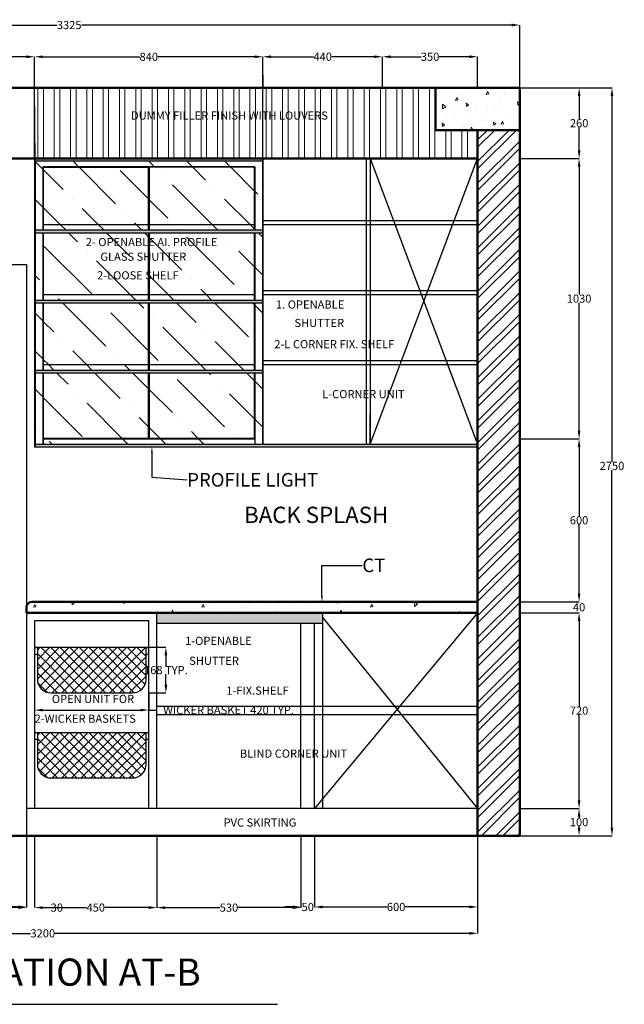
# Model space of a CAD drawing. Units: millimetres. Extents: x 26138 to 44889, y 15820 to 21179.
# Tile 6 of 8: x 37898 to 40122, y 15889 to 19510. Entities that reach past the tile are written whole.
import ezdxf
from ezdxf import colors
from ezdxf.entities.mleader import LeaderData, LeaderLine
from ezdxf.math import Vec2, Vec3

# ---------------------------------------------------------------- set-up
doc = ezdxf.new("R2010")
doc.units = ezdxf.units.MM
doc.header["$MEASUREMENT"] = 0
doc.header["$PDMODE"] = 3
for name, color, linetype, lineweight in [('A-ANNO-DIMS', 70, 'Continuous', 18), ('A-ANNO-SYMB', 1, 'Continuous', 18), ('A-ANNO-TEXT', 7, 'Continuous', 18), ('A-ELEV', 7, 'Continuous', 25), ('A-FURN-PATT', 40, 'Continuous', 13), ('A-WALL', 1, 'Continuous', 50), ('A-WALL-PATT', 8, 'Continuous', 13)]:
    doc.layers.add(name, color=color, linetype=linetype, lineweight=lineweight)
doc.styles.get("Standard").update_dxf_attribs({"font": 'arial.ttf'})
doc.dimstyles.get("Standard").update_dxf_attribs({"dimtxt": 30, "dimasz": 30, "dimexe": 0.18, "dimexo": 0.0625, "dimgap": 0.09, "dimtad": 0, "dimtih": 1, "dimtoh": 1, "dimdec": 0, "dimzin": 0, "dimdsep": 46, "dimtxsty": 'Standard', "dimcen": 0.09, "dimadec": 0, "dimazin": 0, "dimtfac": 1, "dimtdec": 0, "dimtofl": 0, "dimtmove": 0, "dimatfit": 3, "dimfxl": 1, "dimtolj": 1, "dimtzin": 0, "dimarcsym": 0})
pattern_1 = [(95, (-15.19, -1836.28), (88.24832, 74.04913), [12, -132]), (40, (-15.19, -1836.28), (-100.79875, 69.4029), [9.6, -105.6]), (145.45144, (-7.83, -1830.11), (-12.55043, 143.45204), [10.19843, -112.18274]), (91.1842, (-37.81, -1813.65), (139.47094, 102.0182), [18, -198]), (141.63564, (-26.19, -1805.15), (-4.464, 215.95387), [15.29765, -168.2742]), (36.18416, (-37.81, -1813.65), (-4.464, 215.9539), [14.4, -158.4]), (66, (-20.84, -1808), (113.08345, 21.9812), [12, -132]), (11, (-20.84, -1808), (-54.51337, 109.56935), [9.6, -105.6]), (116.45144, (-11.42, -1806.17), (58.57008, 131.55054), [10.19843, -112.18274]), (82.5, (-15.186, -1836.282), (-36.28691, 39.03837), [0, -104.32, 0, -107.2, 0, -106]), (52.5, (-15.186, -1836.28), (-14.85967, 74.38551), [0, -61.12, 0, -101.92, 0, -40.4]), (12.5, (-40.416, -1861.51), (62.946907, 57.84332), [0, -40, 0, -124.8, 0, -165.6]), (2.5, (-51.73, -1872.826), (54.6544, 77.30557), [0, -52, 0, -82.88, 0, -117.6])]
pattern_2 = [(135, (-15.19, -1836.28), (-192.02369, 52.3701), [246.875, -49.375, 0, -49.375])]

# ---------------------------------------------------------------- blocks, each defined once
blk = doc.blocks.new('*D73')
at = {"layer": 'A-ANNO-DIMS', "color": 0, "lineweight": -2, "transparency": 16777216}
for p, q in [((37102.5, 16508.7), (37102.5, 16246.8)), ((37922.5, 16508.7), (37922.5, 16246.8)), ((37132.5, 16247), (37479.3, 16247)), ((37892.5, 16247), (37545.7, 16247))]:
    blk.add_line(p, q, dxfattribs=at)
at = {"layer": 'A-ANNO-DIMS', "color": 0, "transparency": 16777216}
for points in [[(37132.5, 16252), (37132.5, 16242), (37102.5, 16247)], [(37892.5, 16252), (37892.5, 16242), (37922.5, 16247)]]:
    blk.add_solid(points, dxfattribs=at)
at = {"layer": 'Defpoints', "color": 0, "transparency": 16777216}
for p in [(37102.5, 16508.8), (37922.5, 16508.8), (37922.5, 16247)]:
    blk.add_point(p, dxfattribs=at)
at = {"layer": 'A-ANNO-DIMS', "color": 0, "transparency": 16777216, "insert": (37512.5, 16247), "char_height": 30, "attachment_point": 5}
blk.add_mtext('\\A1;820', dxfattribs=at)
blk = doc.blocks.new('*D74')
at = {"layer": 'A-ANNO-DIMS', "color": 0, "lineweight": -2, "transparency": 16777216}
for p, q in [((37922.5, 16508.7), (37922.5, 16244.3)), ((37952.5, 16508.7), (37952.5, 16244.3)), ((37892.5, 16244.5), (37862.5, 16244.5)), ((37982.5, 16244.5), (38012.5, 16244.5))]:
    blk.add_line(p, q, dxfattribs=at)
at = {"layer": 'A-ANNO-DIMS', "color": 0, "transparency": 16777216}
for points in [[(37892.5, 16249.5), (37892.5, 16239.5), (37922.5, 16244.5)], [(37982.5, 16249.5), (37982.5, 16239.5), (37952.5, 16244.5)]]:
    blk.add_solid(points, dxfattribs=at)
at = {"layer": 'Defpoints', "color": 0, "transparency": 16777216}
for p in [(37922.5, 16508.8), (37952.5, 16508.8), (37952.5, 16244.5)]:
    blk.add_point(p, dxfattribs=at)
at = {"layer": 'A-ANNO-DIMS', "color": 0, "transparency": 16777216, "insert": (38034.1, 16244.5), "char_height": 30, "attachment_point": 5}
blk.add_mtext('\\A1;30', dxfattribs=at)
blk = doc.blocks.new('*D75')
at = {"layer": 'A-ANNO-DIMS', "color": 0, "lineweight": -2, "transparency": 16777216}
for p, q in [((37952.5, 16508.7), (37952.5, 16244.3)), ((38402.5, 16508.7), (38402.5, 16244.3)), ((37982.5, 16244.5), (38143.8, 16244.5)), ((38372.5, 16244.5), (38211.3, 16244.5))]:
    blk.add_line(p, q, dxfattribs=at)
at = {"layer": 'A-ANNO-DIMS', "color": 0, "transparency": 16777216}
for points in [[(37982.5, 16249.5), (37982.5, 16239.5), (37952.5, 16244.5)], [(38372.5, 16249.5), (38372.5, 16239.5), (38402.5, 16244.5)]]:
    blk.add_solid(points, dxfattribs=at)
at = {"layer": 'Defpoints', "color": 0, "transparency": 16777216}
for p in [(37952.5, 16508.8), (38402.5, 16508.8), (38402.5, 16244.5)]:
    blk.add_point(p, dxfattribs=at)
at = {"layer": 'A-ANNO-DIMS', "color": 0, "transparency": 16777216, "insert": (38177.5, 16244.5), "char_height": 30, "attachment_point": 5}
blk.add_mtext('\\A1;450', dxfattribs=at)
blk = doc.blocks.new('*D76')
at = {"layer": 'A-ANNO-DIMS', "color": 0, "lineweight": -2, "transparency": 16777216}
for p, q in [((38402.5, 16508.7), (38402.5, 16244.1)), ((38932.5, 16508.7), (38932.5, 16244.1)), ((38432.5, 16244.3), (38634.4, 16244.3)), ((38902.5, 16244.3), (38700.7, 16244.3))]:
    blk.add_line(p, q, dxfattribs=at)
at = {"layer": 'A-ANNO-DIMS', "color": 0, "transparency": 16777216}
for points in [[(38432.5, 16249.3), (38432.5, 16239.3), (38402.5, 16244.3)], [(38902.5, 16249.3), (38902.5, 16239.3), (38932.5, 16244.3)]]:
    blk.add_solid(points, dxfattribs=at)
at = {"layer": 'Defpoints', "color": 0, "transparency": 16777216}
for p in [(38402.5, 16508.8), (38932.5, 16508.8), (38932.5, 16244.3)]:
    blk.add_point(p, dxfattribs=at)
at = {"layer": 'A-ANNO-DIMS', "color": 0, "transparency": 16777216, "insert": (38667.5, 16244.3), "char_height": 30, "attachment_point": 5}
blk.add_mtext('\\A1;530', dxfattribs=at)
blk = doc.blocks.new('*D77')
at = {"layer": 'A-ANNO-DIMS', "color": 0, "lineweight": -2, "transparency": 16777216}
for p, q in [((38932.5, 16508.7), (38932.5, 16246.6)), ((38982.5, 16508.7), (38982.5, 16246.6)), ((38902.5, 16246.8), (38872.5, 16246.8)), ((39012.5, 16246.8), (39042.5, 16246.8))]:
    blk.add_line(p, q, dxfattribs=at)
at = {"layer": 'A-ANNO-DIMS', "color": 0, "transparency": 16777216}
for points in [[(38902.5, 16251.8), (38902.5, 16241.8), (38932.5, 16246.8)], [(39012.5, 16251.8), (39012.5, 16241.8), (38982.5, 16246.8)]]:
    blk.add_solid(points, dxfattribs=at)
at = {"layer": 'Defpoints', "color": 0, "transparency": 16777216}
for p in [(38932.5, 16508.8), (38982.5, 16508.8), (38982.5, 16246.8)]:
    blk.add_point(p, dxfattribs=at)
at = {"layer": 'A-ANNO-DIMS', "color": 0, "transparency": 16777216, "insert": (38957.5, 16246.8), "char_height": 30, "attachment_point": 5}
blk.add_mtext('\\A1;50', dxfattribs=at)
blk = doc.blocks.new('*D78')
at = {"layer": 'A-ANNO-DIMS', "color": 0, "lineweight": -2, "transparency": 16777216}
for p, q in [((38982.5, 16508.7), (38982.5, 16246.6)), ((39582.5, 16508.7), (39582.5, 16246.6)), ((39012.5, 16246.8), (39249.3, 16246.8)), ((39552.5, 16246.8), (39315.8, 16246.8))]:
    blk.add_line(p, q, dxfattribs=at)
at = {"layer": 'A-ANNO-DIMS', "color": 0, "transparency": 16777216}
for points in [[(39012.5, 16251.8), (39012.5, 16241.8), (38982.5, 16246.8)], [(39552.5, 16251.8), (39552.5, 16241.8), (39582.5, 16246.8)]]:
    blk.add_solid(points, dxfattribs=at)
at = {"layer": 'Defpoints', "color": 0, "transparency": 16777216}
for p in [(38982.5, 16508.8), (39582.5, 16508.8), (39582.5, 16246.8)]:
    blk.add_point(p, dxfattribs=at)
at = {"layer": 'A-ANNO-DIMS', "color": 0, "transparency": 16777216, "insert": (39282.5, 16246.8), "char_height": 30, "attachment_point": 5}
blk.add_mtext('\\A1;600', dxfattribs=at)
blk = doc.blocks.new('*D79')
at = {"layer": 'A-ANNO-DIMS', "color": 0, "lineweight": -2, "transparency": 16777216}
for p, q in [((39737.6, 19258.8), (39956.1, 19258.8)), ((39955.9, 19228.8), (39955.9, 19144.2)), ((39955.9, 19028.8), (39955.9, 19113.4)), ((39737.6, 18998.8), (39956.1, 18998.8))]:
    blk.add_line(p, q, dxfattribs=at)
at = {"layer": 'A-ANNO-DIMS', "color": 0, "transparency": 16777216}
for points in [[(39950.9, 19228.8), (39960.9, 19228.8), (39955.9, 19258.8)], [(39950.9, 19028.8), (39960.9, 19028.8), (39955.9, 18998.8)]]:
    blk.add_solid(points, dxfattribs=at)
at = {"layer": 'Defpoints', "color": 0, "transparency": 16777216}
for p in [(39737.5, 19258.8), (39737.5, 18998.8), (39955.9, 18998.8)]:
    blk.add_point(p, dxfattribs=at)
at = {"layer": 'A-ANNO-DIMS', "color": 0, "transparency": 16777216, "insert": (39955.9, 19128.8), "char_height": 30, "attachment_point": 5}
blk.add_mtext('\\A1;260', dxfattribs=at)
blk = doc.blocks.new('*D80')
at = {"layer": 'A-ANNO-DIMS', "color": 0, "lineweight": -2, "transparency": 16777216}
for p, q in [((39737.6, 18998.8), (39955.9, 18998.8)), ((39955.7, 18968.8), (39955.7, 18499.2)), ((39955.7, 17998.8), (39955.7, 18468.3)), ((39737.6, 17968.8), (39955.9, 17968.8))]:
    blk.add_line(p, q, dxfattribs=at)
at = {"layer": 'A-ANNO-DIMS', "color": 0, "transparency": 16777216}
for points in [[(39950.7, 18968.8), (39960.7, 18968.8), (39955.7, 18998.8)], [(39950.7, 17998.8), (39960.7, 17998.8), (39955.7, 17968.8)]]:
    blk.add_solid(points, dxfattribs=at)
at = {"layer": 'Defpoints', "color": 0, "transparency": 16777216}
for p in [(39737.5, 18998.8), (39737.5, 17968.8), (39955.7, 17968.8)]:
    blk.add_point(p, dxfattribs=at)
at = {"layer": 'A-ANNO-DIMS', "color": 0, "transparency": 16777216, "insert": (39955.7, 18483.8), "char_height": 30, "attachment_point": 5}
blk.add_mtext('\\A1;1030', dxfattribs=at)
blk = doc.blocks.new('*D81')
at = {"layer": 'A-ANNO-DIMS', "color": 0, "lineweight": -2, "transparency": 16777216}
for p, q in [((39737.6, 17968.8), (39955.9, 17968.8)), ((39955.7, 17938.8), (39955.7, 17684.2)), ((39955.7, 17398.8), (39955.7, 17653.4)), ((39737.6, 17368.8), (39955.9, 17368.8))]:
    blk.add_line(p, q, dxfattribs=at)
at = {"layer": 'A-ANNO-DIMS', "color": 0, "transparency": 16777216}
for points in [[(39950.7, 17938.8), (39960.7, 17938.8), (39955.7, 17968.8)], [(39950.7, 17398.8), (39960.7, 17398.8), (39955.7, 17368.8)]]:
    blk.add_solid(points, dxfattribs=at)
at = {"layer": 'Defpoints', "color": 0, "transparency": 16777216}
for p in [(39737.5, 17968.8), (39737.5, 17368.8), (39955.7, 17368.8)]:
    blk.add_point(p, dxfattribs=at)
at = {"layer": 'A-ANNO-DIMS', "color": 0, "transparency": 16777216, "insert": (39955.7, 17668.8), "char_height": 30, "attachment_point": 5}
blk.add_mtext('\\A1;600', dxfattribs=at)
blk = doc.blocks.new('*D82')
at = {"layer": 'A-ANNO-DIMS', "color": 0, "lineweight": -2, "transparency": 16777216}
for p, q in [((39955.7, 17398.8), (39955.7, 17428.8)), ((39737.6, 17368.8), (39955.9, 17368.8)), ((39737.6, 17328.8), (39955.9, 17328.8)), ((39955.7, 17298.8), (39955.7, 17268.8))]:
    blk.add_line(p, q, dxfattribs=at)
at = {"layer": 'A-ANNO-DIMS', "color": 0, "transparency": 16777216}
for points in [[(39950.7, 17398.8), (39960.7, 17398.8), (39955.7, 17368.8)], [(39950.7, 17298.8), (39960.7, 17298.8), (39955.7, 17328.8)]]:
    blk.add_solid(points, dxfattribs=at)
at = {"layer": 'Defpoints', "color": 0, "transparency": 16777216}
for p in [(39737.5, 17368.8), (39737.5, 17328.8), (39955.7, 17328.8)]:
    blk.add_point(p, dxfattribs=at)
at = {"layer": 'A-ANNO-DIMS', "color": 0, "transparency": 16777216, "insert": (39955.7, 17348.8), "char_height": 30, "attachment_point": 5}
blk.add_mtext('\\A1;40', dxfattribs=at)
blk = doc.blocks.new('*D83')
at = {"layer": 'A-ANNO-DIMS', "color": 0, "lineweight": -2, "transparency": 16777216}
for p, q in [((39737.6, 17328.8), (39955.9, 17328.8)), ((39955.7, 17298.8), (39955.7, 16984.2)), ((39955.7, 16638.8), (39955.7, 16953.4)), ((39737.6, 16608.8), (39955.9, 16608.8))]:
    blk.add_line(p, q, dxfattribs=at)
at = {"layer": 'A-ANNO-DIMS', "color": 0, "transparency": 16777216}
for points in [[(39950.7, 17298.8), (39960.7, 17298.8), (39955.7, 17328.8)], [(39950.7, 16638.8), (39960.7, 16638.8), (39955.7, 16608.8)]]:
    blk.add_solid(points, dxfattribs=at)
at = {"layer": 'Defpoints', "color": 0, "transparency": 16777216}
for p in [(39737.5, 17328.8), (39737.5, 16608.8), (39955.7, 16608.8)]:
    blk.add_point(p, dxfattribs=at)
at = {"layer": 'A-ANNO-DIMS', "color": 0, "transparency": 16777216, "insert": (39955.7, 16968.8), "char_height": 30, "attachment_point": 5}
blk.add_mtext('\\A1;720', dxfattribs=at)
blk = doc.blocks.new('*D84')
at = {"layer": 'A-ANNO-DIMS', "color": 0, "lineweight": -2, "transparency": 16777216}
for p, q in [((39737.6, 16608.8), (39955.7, 16608.8)), ((39955.6, 16578.8), (39955.6, 16574.2)), ((39955.6, 16538.8), (39955.6, 16543.4)), ((39737.6, 16508.8), (39955.7, 16508.8))]:
    blk.add_line(p, q, dxfattribs=at)
at = {"layer": 'A-ANNO-DIMS', "color": 0, "transparency": 16777216}
for points in [[(39950.6, 16578.8), (39960.6, 16578.8), (39955.6, 16608.8)], [(39950.6, 16538.8), (39960.6, 16538.8), (39955.6, 16508.8)]]:
    blk.add_solid(points, dxfattribs=at)
at = {"layer": 'Defpoints', "color": 0, "transparency": 16777216}
for p in [(39737.5, 16608.8), (39737.5, 16508.8), (39955.6, 16508.8)]:
    blk.add_point(p, dxfattribs=at)
at = {"layer": 'A-ANNO-DIMS', "color": 0, "transparency": 16777216, "insert": (39955.6, 16558.8), "char_height": 30, "attachment_point": 5}
blk.add_mtext('\\A1;100', dxfattribs=at)
blk = doc.blocks.new('*D88')
at = {"layer": 'A-ANNO-DIMS', "color": 0, "lineweight": -2, "transparency": 16777216}
for p, q in [((36732.5, 19258.8), (36732.5, 19373.3)), ((36762.5, 19373.2), (37299.1, 19373.2)), ((37922.5, 19373.2), (37386, 19373.2)), ((37952.5, 19258.8), (37952.5, 19373.3))]:
    blk.add_line(p, q, dxfattribs=at)
at = {"layer": 'A-ANNO-DIMS', "color": 0, "transparency": 16777216}
for points in [[(36762.5, 19378.2), (36762.5, 19368.2), (36732.5, 19373.2)], [(37922.5, 19378.2), (37922.5, 19368.2), (37952.5, 19373.2)]]:
    blk.add_solid(points, dxfattribs=at)
at = {"layer": 'Defpoints', "color": 0, "transparency": 16777216}
for p in [(37952.5, 19373.2), (36732.5, 19258.8), (37952.5, 19258.8)]:
    blk.add_point(p, dxfattribs=at)
at = {"layer": 'A-ANNO-DIMS', "color": 0, "transparency": 16777216, "insert": (37342.5, 19373.2), "char_height": 30, "attachment_point": 5}
blk.add_mtext('\\A1;1220', dxfattribs=at)
blk = doc.blocks.new('*D89')
at = {"layer": 'A-ANNO-DIMS', "color": 0, "lineweight": -2, "transparency": 16777216}
for p, q in [((37952.5, 18998.8), (37952.5, 19373.3)), ((37982.5, 19373.2), (38339.3, 19373.2)), ((38762.5, 19373.2), (38405.7, 19373.2)), ((38792.5, 18998.8), (38792.5, 19373.3))]:
    blk.add_line(p, q, dxfattribs=at)
at = {"layer": 'A-ANNO-DIMS', "color": 0, "transparency": 16777216}
for points in [[(37982.5, 19378.2), (37982.5, 19368.2), (37952.5, 19373.2)], [(38762.5, 19378.2), (38762.5, 19368.2), (38792.5, 19373.2)]]:
    blk.add_solid(points, dxfattribs=at)
at = {"layer": 'Defpoints', "color": 0, "transparency": 16777216}
for p in [(38792.5, 19373.2), (37952.5, 18998.8), (38792.5, 18998.8)]:
    blk.add_point(p, dxfattribs=at)
at = {"layer": 'A-ANNO-DIMS', "color": 0, "transparency": 16777216, "insert": (38372.5, 19373.2), "char_height": 30, "attachment_point": 5}
blk.add_mtext('\\A1;840', dxfattribs=at)
blk = doc.blocks.new('*D90')
at = {"layer": 'A-ANNO-DIMS', "color": 0, "lineweight": -2, "transparency": 16777216}
for p, q in [((38792.5, 19258.8), (38792.5, 19373.5)), ((38822.5, 19373.3), (38978.8, 19373.3)), ((39202.5, 19373.3), (39046.3, 19373.3)), ((39232.5, 19258.8), (39232.5, 19373.5))]:
    blk.add_line(p, q, dxfattribs=at)
at = {"layer": 'A-ANNO-DIMS', "color": 0, "transparency": 16777216}
for points in [[(38822.5, 19378.3), (38822.5, 19368.3), (38792.5, 19373.3)], [(39202.5, 19378.3), (39202.5, 19368.3), (39232.5, 19373.3)]]:
    blk.add_solid(points, dxfattribs=at)
at = {"layer": 'Defpoints', "color": 0, "transparency": 16777216}
for p in [(39232.5, 19373.3), (38792.5, 19258.8), (39232.5, 19258.8)]:
    blk.add_point(p, dxfattribs=at)
at = {"layer": 'A-ANNO-DIMS', "color": 0, "transparency": 16777216, "insert": (39012.5, 19373.3), "char_height": 30, "attachment_point": 5}
blk.add_mtext('\\A1;440', dxfattribs=at)
blk = doc.blocks.new('*D91')
at = {"layer": 'A-ANNO-DIMS', "color": 0, "lineweight": -2, "transparency": 16777216}
for p, q in [((39232.5, 19258.8), (39232.5, 19373.5)), ((39262.5, 19373.3), (39374.4, 19373.3)), ((39552.5, 19373.3), (39440.7, 19373.3)), ((39582.5, 19258.8), (39582.5, 19373.5))]:
    blk.add_line(p, q, dxfattribs=at)
at = {"layer": 'A-ANNO-DIMS', "color": 0, "transparency": 16777216}
for points in [[(39262.5, 19378.3), (39262.5, 19368.3), (39232.5, 19373.3)], [(39552.5, 19378.3), (39552.5, 19368.3), (39582.5, 19373.3)]]:
    blk.add_solid(points, dxfattribs=at)
at = {"layer": 'Defpoints', "color": 0, "transparency": 16777216}
for p in [(39582.5, 19373.3), (39232.5, 19258.8), (39582.5, 19258.8)]:
    blk.add_point(p, dxfattribs=at)
at = {"layer": 'A-ANNO-DIMS', "color": 0, "transparency": 16777216, "insert": (39407.5, 19373.3), "char_height": 30, "attachment_point": 5}
blk.add_mtext('\\A1;350', dxfattribs=at)
blk = doc.blocks.new('*D92')
at = {"layer": 'A-ANNO-DIMS', "color": 0, "lineweight": -2, "transparency": 16777216}
for p, q in [((36382.5, 16509), (36382.5, 16149.6)), ((39582.5, 16508.7), (39582.5, 16149.6)), ((36412.5, 16149.8), (37937.7, 16149.8)), ((39552.5, 16149.8), (38027.4, 16149.8))]:
    blk.add_line(p, q, dxfattribs=at)
at = {"layer": 'A-ANNO-DIMS', "color": 0, "transparency": 16777216}
for points in [[(36412.5, 16154.8), (36412.5, 16144.8), (36382.5, 16149.8)], [(39552.5, 16154.8), (39552.5, 16144.8), (39582.5, 16149.8)]]:
    blk.add_solid(points, dxfattribs=at)
at = {"layer": 'Defpoints', "color": 0, "transparency": 16777216}
for p in [(36382.5, 16509), (39582.5, 16508.8), (39582.5, 16149.8)]:
    blk.add_point(p, dxfattribs=at)
at = {"layer": 'A-ANNO-DIMS', "color": 0, "transparency": 16777216, "insert": (37982.5, 16149.8), "char_height": 30, "attachment_point": 5}
blk.add_mtext('\\A1;3200', dxfattribs=at)
blk = doc.blocks.new('*D117')
at = {"layer": 'A-ANNO-DIMS', "color": 0, "lineweight": -2, "transparency": 16777216}
for p, q in [((39737.6, 19258.8), (40076.9, 19258.8)), ((40076.7, 19228.8), (40076.7, 17884.2)), ((40076.7, 16538.8), (40076.7, 17853.3)), ((39737.6, 16508.8), (40076.9, 16508.8))]:
    blk.add_line(p, q, dxfattribs=at)
at = {"layer": 'A-ANNO-DIMS', "color": 0, "transparency": 16777216}
for points in [[(40071.7, 19228.8), (40081.7, 19228.8), (40076.7, 19258.8)], [(40071.7, 16538.8), (40081.7, 16538.8), (40076.7, 16508.8)]]:
    blk.add_solid(points, dxfattribs=at)
at = {"layer": 'Defpoints', "color": 0, "transparency": 16777216}
for p in [(39737.5, 19258.8), (39737.5, 16508.8), (40076.7, 16508.8)]:
    blk.add_point(p, dxfattribs=at)
at = {"layer": 'A-ANNO-DIMS', "color": 0, "transparency": 16777216, "insert": (40076.7, 17868.7), "char_height": 30, "attachment_point": 5}
blk.add_mtext('\\A1;2750', dxfattribs=at)
blk = doc.blocks.new('*D118')
at = {"layer": 'A-ANNO-DIMS', "color": 0, "lineweight": -2, "transparency": 16777216}
for p, q in [((36412.5, 19258.8), (36412.5, 19490)), ((36442.5, 19489.9), (38034.6, 19489.9)), ((39707.5, 19489.9), (38124.6, 19489.9)), ((39737.5, 19258.8), (39737.5, 19490))]:
    blk.add_line(p, q, dxfattribs=at)
at = {"layer": 'A-ANNO-DIMS', "color": 0, "transparency": 16777216}
for points in [[(36442.5, 19494.9), (36442.5, 19484.9), (36412.5, 19489.9)], [(39707.5, 19494.9), (39707.5, 19484.9), (39737.5, 19489.9)]]:
    blk.add_solid(points, dxfattribs=at)
at = {"layer": 'Defpoints', "color": 0, "transparency": 16777216}
for p in [(39737.5, 19489.9), (36412.5, 19258.8), (39737.5, 19258.8)]:
    blk.add_point(p, dxfattribs=at)
at = {"layer": 'A-ANNO-DIMS', "color": 0, "transparency": 16777216, "insert": (38079.6, 19489.9), "char_height": 30, "attachment_point": 5}
blk.add_mtext('\\A1;3325', dxfattribs=at)
blk = doc.blocks.new('WICKER-BASKET')
for p, q in [((0, 167.7), (10, 167.7)), ((10, 167.7), (10, 50)), ((410, 50), (410, 167.7)), ((410, 167.7), (420, 167.7)), ((60, 0), (360, 0))]:
    blk.add_line(p, q)
for centre, start, end in [((60, 50), 180, 270), ((360, 50), 270, 0)]:
    blk.add_arc(centre, 50, start, end)
blk = doc.blocks.new('*D129')
at = {"layer": 'A-ANNO-DIMS', "color": 0, "lineweight": -2, "transparency": 16777216}
for p, q in [((37952.5, 17033.7), (37952.5, 16970.6)), ((38372.5, 17033.7), (38372.5, 16970.6)), ((37982.5, 16970.8), (38342.5, 16970.8)), ((38372.5, 16970.8), (38402.5, 16970.8))]:
    blk.add_line(p, q, dxfattribs=at)
at = {"layer": 'A-ANNO-DIMS', "color": 0, "transparency": 16777216}
for points in [[(37982.5, 16975.8), (37982.5, 16965.8), (37952.5, 16970.8)], [(38342.5, 16975.8), (38342.5, 16965.8), (38372.5, 16970.8)]]:
    blk.add_solid(points, dxfattribs=at)
at = {"layer": 'Defpoints', "color": 0, "transparency": 16777216}
for p in [(37952.5, 17033.8), (38372.5, 17033.8), (38372.5, 16970.8)]:
    blk.add_point(p, dxfattribs=at)
at = {"layer": 'A-ANNO-DIMS', "color": 0, "transparency": 16777216, "insert": (38666.1, 16970.8), "char_height": 30, "attachment_point": 5}
blk.add_mtext('\\A1;WICKER BASKET 420 TYP.', dxfattribs=at)
blk = doc.blocks.new('*D130')
at = {"layer": 'A-ANNO-DIMS', "color": 0, "lineweight": -2, "transparency": 16777216}
for p, q in [((38372.6, 17201.6), (38435.7, 17201.6)), ((38435.5, 17171.6), (38435.5, 17133.1)), ((38435.5, 17063.8), (38435.5, 17102.3)), ((38372.6, 17033.8), (38435.7, 17033.8))]:
    blk.add_line(p, q, dxfattribs=at)
at = {"layer": 'A-ANNO-DIMS', "color": 0, "transparency": 16777216}
for points in [[(38430.5, 17171.6), (38440.5, 17171.6), (38435.5, 17201.6)], [(38430.5, 17063.8), (38440.5, 17063.8), (38435.5, 17033.8)]]:
    blk.add_solid(points, dxfattribs=at)
at = {"layer": 'Defpoints', "color": 0, "transparency": 16777216}
for p in [(38372.5, 17201.6), (38435.5, 17201.6), (38372.5, 17033.8)]:
    blk.add_point(p, dxfattribs=at)
at = {"layer": 'A-ANNO-DIMS', "color": 0, "transparency": 16777216, "insert": (38435.5, 17117.7), "char_height": 30, "attachment_point": 5}
blk.add_mtext('\\A1;168 TYP.', dxfattribs=at)

msp = doc.modelspace()

# ---------------------------------------------------------------- hatches: boundary and pattern name
at = {"layer": 'A-FURN-PATT'}
h = msp.add_hatch(color=256, dxfattribs=at)
h.dxf.hatch_style = 1
h.paths.add_polyline_path([(38792.548, 18988.766), (38792.548, 18998.766), (37952.548, 18998.766), (37952.548, 18988.766)])
h = msp.add_hatch(dxfattribs=at)
h.set_pattern_fill('ANSI36', color=256, scale=790, angle=90)
h.set_pattern_definition(pattern_2)
h.paths.add_polyline_path([(37982.548, 18968.766), (38762.548, 18968.766), (38762.548, 18736.288), (38790.548, 18736.288), (38790.548, 18988.766), (37954.548, 18988.766), (37954.548, 18736.288), (37982.548, 18736.288)])
h = msp.add_hatch(dxfattribs=at)
h.set_pattern_fill('ANSI36', color=256, scale=790, angle=90)
h.set_pattern_definition(pattern_2)
h.paths.add_polyline_path([(37984.548, 18966.766), (37984.548, 18756.266), (38370.548, 18756.266), (38370.548, 18966.766)], flags=17)
h = msp.add_hatch(dxfattribs=at)
h.set_pattern_fill('ANSI36', color=256, scale=790, angle=90)
h.set_pattern_definition(pattern_2)
h.paths.add_polyline_path([(38374.548, 18966.766), (38374.548, 18756.266), (38760.548, 18756.266), (38760.548, 18966.766)], flags=17)
h = msp.add_hatch(dxfattribs=at)
h.set_pattern_fill('ANSI36', color=256, scale=790, angle=90)
h.set_pattern_definition(pattern_2)
h.paths.add_polyline_path([(38370.548, 18756.266), (37984.548, 18756.266), (37984.548, 18736.288), (38370.548, 18736.288)], flags=17)
h = msp.add_hatch(dxfattribs=at)
h.set_pattern_fill('ANSI36', color=256, scale=790, angle=90)
h.set_pattern_definition(pattern_2)
h.paths.add_polyline_path([(38760.548, 18756.266), (38374.548, 18756.266), (38374.548, 18736.288), (38760.548, 18736.288)], flags=17)
h = msp.add_hatch(color=256, dxfattribs=at)
h.dxf.hatch_style = 1
h.paths.add_polyline_path([(37952.548, 18736.288), (37952.548, 18726.266), (38792.548, 18726.266), (38792.548, 18736.288)])
h = msp.add_hatch(dxfattribs=at)
h.set_pattern_fill('ANSI36', color=256, scale=790, angle=90)
h.set_pattern_definition(pattern_2)
h.paths.add_polyline_path([(37982.548, 18726.266), (37954.548, 18726.266), (37954.548, 18478.766), (37982.548, 18478.766)])
h = msp.add_hatch(dxfattribs=at)
h.set_pattern_fill('ANSI36', color=256, scale=790, angle=90)
h.set_pattern_definition(pattern_2)
h.paths.add_polyline_path([(38370.548, 18498.766), (38370.548, 18726.266), (37984.548, 18726.266), (37984.548, 18498.766)])
h = msp.add_hatch(dxfattribs=at)
h.set_pattern_fill('ANSI36', color=256, scale=790, angle=90)
h.set_pattern_definition(pattern_2)
h.paths.add_polyline_path([(38760.548, 18498.766), (38760.548, 18726.266), (38374.548, 18726.266), (38374.548, 18498.766)])
h = msp.add_hatch(dxfattribs=at)
h.set_pattern_fill('ANSI36', color=256, scale=790, angle=90)
h.set_pattern_definition(pattern_2)
h.paths.add_polyline_path([(38790.548, 18726.266), (38762.548, 18726.266), (38762.548, 18478.766), (38790.548, 18478.766)])
h = msp.add_hatch(color=256, dxfattribs=at)
h.dxf.hatch_style = 1
h.paths.add_polyline_path([(37952.548, 18478.766), (37952.548, 18468.766), (38792.548, 18468.766), (38792.548, 18478.766)])
h = msp.add_hatch(dxfattribs=at)
h.set_pattern_fill('ANSI36', color=256, scale=790, angle=90)
h.set_pattern_definition(pattern_2)
h.paths.add_polyline_path([(37982.548, 18468.766), (37954.548, 18468.766), (37954.548, 18221.266), (37982.548, 18221.266)])
h = msp.add_hatch(dxfattribs=at)
h.set_pattern_fill('ANSI36', color=256, scale=790, angle=90)
h.set_pattern_definition(pattern_2)
h.paths.add_polyline_path([(38370.548, 18498.766), (37984.548, 18498.766), (37984.548, 18478.766), (38370.548, 18478.766)])
h = msp.add_hatch(dxfattribs=at)
h.set_pattern_fill('ANSI36', color=256, scale=790, angle=90)
h.set_pattern_definition(pattern_2)
h.paths.add_polyline_path([(38370.548, 18241.266), (38370.548, 18468.766), (37984.548, 18468.766), (37984.548, 18241.266)])
h = msp.add_hatch(dxfattribs=at)
h.set_pattern_fill('ANSI36', color=256, scale=790, angle=90)
h.set_pattern_definition(pattern_2)
h.paths.add_polyline_path([(38760.548, 18498.766), (38374.548, 18498.766), (38374.548, 18478.766), (38760.548, 18478.766)])
h = msp.add_hatch(dxfattribs=at)
h.set_pattern_fill('ANSI36', color=256, scale=790, angle=90)
h.set_pattern_definition(pattern_2)
h.paths.add_polyline_path([(38374.548, 18468.766), (38374.548, 18241.266), (38760.548, 18241.266), (38760.548, 18468.766)])
h = msp.add_hatch(dxfattribs=at)
h.set_pattern_fill('ANSI36', color=256, scale=790, angle=90)
h.set_pattern_definition(pattern_2)
h.paths.add_polyline_path([(38790.548, 18468.766), (38762.548, 18468.766), (38762.548, 18221.266), (38790.548, 18221.266)])
h = msp.add_hatch(color=256, dxfattribs=at)
h.dxf.hatch_style = 1
h.paths.add_polyline_path([(38792.548, 18211.266), (38792.548, 18221.266), (37952.548, 18221.266), (37952.548, 18211.266)])
h = msp.add_hatch(dxfattribs=at)
h.set_pattern_fill('ANSI36', color=256, scale=790, angle=90)
h.set_pattern_definition(pattern_2)
h.paths.add_polyline_path([(38370.548, 18241.266), (37984.548, 18241.266), (37984.548, 18221.266), (38370.548, 18221.266)])
h = msp.add_hatch(dxfattribs=at)
h.set_pattern_fill('ANSI36', color=256, scale=790, angle=90)
h.set_pattern_definition(pattern_2)
h.paths.add_polyline_path([(38760.548, 18241.266), (38374.548, 18241.266), (38374.548, 18221.266), (38760.548, 18221.266)])
h = msp.add_hatch(dxfattribs=at)
h.set_pattern_fill('ANSI36', color=256, scale=790, angle=90)
h.set_pattern_definition(pattern_2)
h.paths.add_polyline_path([(37982.548, 18211.266), (37954.548, 18211.266), (37954.548, 17948.766), (37982.548, 17948.766)])
h = msp.add_hatch(dxfattribs=at)
h.set_pattern_fill('ANSI36', color=256, scale=790, angle=90)
h.set_pattern_definition(pattern_2)
h.paths.add_polyline_path([(37984.548, 18211.266), (37984.548, 17970.766), (38370.548, 17970.766), (38370.548, 18211.266)])
h = msp.add_hatch(dxfattribs=at)
h.set_pattern_fill('ANSI36', color=256, scale=790, angle=90)
h.set_pattern_definition(pattern_2)
h.paths.add_polyline_path([(38374.548, 18211.266), (38374.548, 17970.766), (38760.548, 17970.766), (38760.548, 18211.266)])
h = msp.add_hatch(dxfattribs=at)
h.set_pattern_fill('ANSI36', color=256, scale=790, angle=90)
h.set_pattern_definition(pattern_2)
h.paths.add_polyline_path([(38790.548, 18211.266), (38762.548, 18211.266), (38762.548, 17948.766), (38790.548, 17948.766)])
h = msp.add_hatch(dxfattribs=at)
h.set_pattern_fill('ANSI36', color=256, scale=790, angle=90)
h.set_pattern_definition(pattern_2)
h.paths.add_polyline_path([(38762.548, 17968.766), (37984.548, 17968.766), (37984.548, 17948.766), (38762.548, 17948.766)])
h = msp.add_hatch(color=256, dxfattribs=at)
h.dxf.hatch_style = 1
h.paths.add_polyline_path([(37952.548, 17948.766), (37952.548, 17938.766), (38792.548, 17938.766), (38792.548, 17948.766)])
h = msp.add_hatch(color=256, dxfattribs=at)
h.dxf.hatch_style = 1
h.paths.add_polyline_path([(39582.548, 17948.766), (37952.548, 17948.766), (37952.548, 17938.766), (39582.548, 17938.766)])
h = msp.add_hatch(color=256, dxfattribs=at)
h.dxf.hatch_style = 1
h.paths.add_polyline_path([(39552.548, 17948.766), (38792.548, 17948.766), (38792.548, 17938.766), (39552.548, 17938.766)])
h = msp.add_hatch(color=256, dxfattribs=at)
h.dxf.hatch_style = 1
h.paths.add_polyline_path([(38402.548, 17328.766), (38402.548, 17288.766), (39012.548, 17288.766), (39012.548, 17328.766)])
h = msp.add_hatch(dxfattribs=at)
h.set_pattern_fill('ANSI37', color=256, scale=200, angle=90)
h.set_pattern_definition([(135, (-15.186, -1836.282), (-17.67767, -17.67767), []), (225, (-15.186, -1836.282), (17.67767, -17.67767), [])])
h.paths.add_polyline_path([(38312.548, 17033.811, 0.41421356), (38362.548, 17083.811), (38362.548, 17201.557), (37962.548, 17201.557), (37962.548, 17083.811, 0.41421356), (38012.548, 17033.811)])
h = msp.add_hatch(dxfattribs=at)
h.set_pattern_fill('ANSI37', color=256, scale=200, angle=90)
h.set_pattern_definition([(135, (-15.186, -2148.976), (-17.67767, -17.67767), []), (225, (-15.186, -2148.976), (17.67767, -17.67767), [])])
h.paths.add_polyline_path([(38312.548, 16721.117, 0.41421356), (38362.548, 16771.117), (38362.548, 16888.863), (37962.548, 16888.863), (37962.548, 16771.117, 0.41421356), (38012.548, 16721.117)])
at = {"layer": 'A-WALL-PATT'}
h = msp.add_hatch(dxfattribs=at)
h.set_pattern_fill('ANSI32', color=256, scale=160, angle=45)
h.set_pattern_definition([(90, (-15.186, -1836.28), (-60, 0), []), (90, (4.814, -1816.28), (-60, 0), [])])
h.paths.add_polyline_path([(37952.548, 19258.766), (37954.474, 18998.766), (39582.548, 18998.766), (39582.548, 19103.766), (39427.548, 19103.766), (39427.548, 19258.766)])
h.paths.add_polyline_path([(38299.413, 19133.795), (39106.641, 19133.795), (39106.641, 19180.36), (38299.413, 19180.36)], flags=24)
h = msp.add_hatch(dxfattribs=at)
h.set_pattern_fill('AR-CONC', color=256, scale=16, angle=45)
h.set_pattern_definition(pattern_1)
h.paths.add_polyline_path([(39737.548, 19103.766), (39737.548, 19258.766), (39427.548, 19258.766), (39427.548, 19103.766)])
h = msp.add_hatch(dxfattribs=at)
h.set_pattern_fill('ANSI32', color=256, scale=150)
h.set_pattern_definition([(45, (-15.186, -1836.28), (-39.774756, 39.774756), []), (45, (11.33, -1836.28), (-39.774756, 39.774756), [])])
h.paths.add_polyline_path([(39737.548, 19103.766), (39582.548, 19103.766), (39582.548, 16508.766), (39737.548, 16508.766)])
h = msp.add_hatch(dxfattribs=at)
h.set_pattern_fill('AR-CONC', color=256, scale=16, angle=45)
h.set_pattern_definition(pattern_1)
h.paths.add_polyline_path([(37942.548, 17368.766, 0.41421356), (37922.548, 17348.766), (37922.548, 17328.766), (38402.548, 17328.766), (39582.548, 17328.766), (39582.548, 17368.766)])

# ---------------------------------------------------------------- linework, layer by layer
at = {"layer": 'A-ANNO-SYMB'}
for p in [(37952.548, 18741.266), (37952.548, 18483.766), (37952.548, 18226.266)]:
    msp.add_point(p, dxfattribs=at)
at = {"layer": 'A-ELEV'}
for p, q in [((38792.548, 19306.068), (38792.548, 19258.766)), ((37954.548, 18988.766), (37952.548, 19258.766)), ((37952.548, 18998.766), (37952.548, 17938.766)), ((38792.548, 18988.766), (37952.548, 18988.766)), ((37954.548, 18998.766), (37954.548, 17938.766)), ((38790.548, 18998.766), (38790.548, 17948.766)), ((38792.548, 18998.766), (38792.548, 17948.766)), ((39172.548, 18998.766), (39172.548, 17948.766)), ((39187.548, 18998.766), (39187.548, 17948.766)), ((39187.548, 18998.766), (39582.548, 17948.766)), ((39187.548, 17948.766), (39582.548, 18998.766)), ((37982.548, 18968.766), (37982.548, 18736.288)), ((38762.548, 18968.766), (37982.548, 18968.766)), ((37984.548, 18966.766), (37984.548, 18736.288)), ((37984.548, 18966.766), (38370.548, 18966.766)), ((38370.548, 18966.766), (38370.548, 18736.266)), ((38374.548, 18966.766), (38374.548, 18736.266)), ((38760.548, 18966.766), (38374.548, 18966.766)), ((38760.548, 18966.766), (38760.548, 18736.288)), ((38762.548, 18968.766), (38762.548, 18736.288)), ((37982.548, 18756.266), (38762.548, 18756.266)), ((38792.548, 18771.266), (39582.548, 18771.266)), ((38792.548, 18756.266), (39582.548, 18756.266)), ((37952.548, 18736.288), (38792.548, 18736.288)), ((37952.548, 18726.266), (38792.548, 18726.266)), ((37982.548, 18726.266), (37982.548, 18478.766)), ((37984.548, 18726.266), (37984.548, 18478.766)), ((38370.548, 18726.266), (38370.548, 18478.766)), ((38374.548, 18726.266), (38374.548, 18478.766)), ((38760.548, 18726.266), (38760.548, 18478.766)), ((38762.548, 18726.266), (38762.548, 18478.766)), ((37102.548, 18608.766), (37922.548, 18608.766)), ((37922.548, 18608.766), (37922.548, 16508.766)), ((38792.548, 18513.766), (39582.548, 18513.766)), ((37952.548, 18478.766), (38792.548, 18478.766)), ((37952.548, 18468.766), (38792.548, 18468.766)), ((37982.548, 18498.766), (38762.548, 18498.766)), ((37982.548, 18468.766), (37982.548, 18221.266)), ((37984.548, 18468.766), (37984.548, 18221.266)), ((38370.548, 18468.766), (38370.548, 18221.266)), ((38374.548, 18468.766), (38374.548, 18221.266)), ((38760.548, 18468.766), (38760.548, 18221.266)), ((38762.548, 18468.766), (38762.548, 18221.266)), ((38792.548, 18498.766), (39582.548, 18498.766)), ((38792.548, 18256.266), (39582.548, 18256.266)), ((37952.548, 18221.266), (38792.548, 18221.266)), ((37982.548, 18241.266), (38762.548, 18241.266)), ((38792.548, 18241.266), (39582.548, 18241.266)), ((37952.548, 18211.266), (38792.548, 18211.266)), ((37982.548, 18211.266), (37982.548, 17948.766)), ((37984.548, 18211.266), (37984.548, 17948.766)), ((38370.548, 18211.266), (38370.548, 17968.766)), ((38374.548, 18211.266), (38374.548, 17968.766)), ((38760.548, 18211.266), (38760.548, 17970.766)), ((38762.548, 18211.266), (38762.548, 17948.766)), ((39187.548, 17948.766), (39187.548, 18057.233)), ((37982.548, 17968.766), (38762.548, 17968.766)), ((37984.548, 17970.766), (38760.548, 17970.766)), ((37952.548, 17948.766), (39582.548, 17948.766)), ((37952.548, 17938.766), (39582.548, 17938.766)), ((39172.548, 17948.766), (39187.548, 17948.766)), ((37922.548, 17313.766), (37922.548, 16608.766)), ((38402.548, 16953.766), (38402.548, 17328.766)), ((39582.548, 17328.766), (38982.548, 16608.766)), ((39012.548, 16608.766), (39012.548, 17328.766)), ((39012.548, 17310.304), (39582.548, 16608.766)), ((37952.548, 17298.766), (37952.548, 16608.766)), ((38372.548, 17298.766), (37952.548, 17298.766)), ((38372.548, 16608.766), (38372.548, 17298.766)), ((39012.548, 17288.766), (38402.548, 17288.766)), ((38932.548, 16608.766), (38932.548, 17288.766)), ((38982.548, 16608.766), (38982.548, 17288.766)), ((37957.548, 17201.557), (38367.548, 17201.557)), ((37952.548, 17176.823), (37962.548, 17176.823)), ((38362.548, 17176.823), (38372.548, 17176.823)), ((38372.548, 17033.811), (38372.548, 17033.811)), ((39582.548, 16983.766), (38402.548, 16983.766)), ((38372.548, 16608.766), (38372.548, 16958.766)), ((38402.548, 16608.766), (38402.548, 16958.766)), ((39582.548, 16953.766), (38402.548, 16953.766)), ((37957.548, 16888.863), (38367.548, 16888.863)), ((37952.548, 16864.129), (37962.548, 16864.129)), ((38362.548, 16864.129), (38372.548, 16864.129)), ((38372.548, 16721.117), (38372.548, 16721.117)), ((39582.548, 16608.766), (37922.548, 16608.766)), ((36832.787, 15888.819), (38846.464, 15888.819))]:
    msp.add_line(p, q, dxfattribs=at)
at = {"layer": 'A-WALL'}
for p, q in [((39737.548, 19258.766), (36109.548, 19258.766)), ((39427.548, 19103.766), (39427.548, 19258.766)), ((39737.548, 16508.766), (39737.548, 19258.766)), ((39737.548, 19258.766), (39737.548, 19103.766)), ((39737.548, 19103.766), (39427.548, 19103.766)), ((39582.548, 16508.766), (39582.548, 19103.766)), ((39582.548, 18998.766), (36109.548, 18998.766)), ((37922.548, 17348.766), (37922.548, 17328.766)), ((39582.548, 17368.766), (37942.548, 17368.766)), ((39582.548, 17328.766), (37922.548, 17328.766)), ((36109.548, 16508.766), (39737.548, 16508.766))]:
    msp.add_line(p, q, dxfattribs=at)
msp.add_arc((37942.548, 17348.766), 20, 90, 180, dxfattribs=at)

# ---------------------------------------------------------------- block references
at = {"layer": 'A-ELEV'}
for p in [(37952.548, 17033.811), (37952.548, 16721.117)]:
    msp.add_blockref('WICKER-BASKET', p, dxfattribs=at)

# ---------------------------------------------------------------- texts
at = {"layer": 'A-ANNO-TEXT'}
for s, height, p in [('DUMMY FILLER FINISH WITH LOUVERS', 30, (38307.174, 19142.067)), ('2- OPENABLE AI. PROFILE', 30, (38140.677, 18676.74)), ('GLASS SHUTTER', 30, (38194.438, 18622.978)), ('2-LOOSE SHELF', 30, (38182.123, 18554.457)), ('1. OPENABLE', 30, (38840.54, 18447.13)), ('SHUTTER', 30, (38908.377, 18379.409)), ('2-L CORNER FIX. SHELF', 30, (38834.352, 18301.377)), ('L-CORNER UNIT', 30, (39010.624, 18117.605)), ('BACK SPLASH', 60, (38723.173, 17658.639)), ('1-OPENABLE', 30, (38506.071, 17210.266)), ('SHUTTER', 30, (38521.321, 17137.114)), ('1-FIX.SHELF', 30, (38657.74, 17027.386)), ('OPEN UNIT FOR ', 30, (38015.758, 16996.744)), ('2-WICKER BASKETS', 30, (37952.548, 16924.235)), ('BLIND CORNER UNIT', 30, (38707.74, 16795.739)), ('PVC SKIRTING', 30, (38647.633, 16542.267)), ('KITCHEN ELEVATION AT-B', 100, (36907.79, 15957.078))]:
    msp.add_text(s, height=height, dxfattribs=at).set_placement(p)

# ---------------------------------------------------------------- dimensions: what is measured, and where the dimension line sits
at = {"layer": 'A-ANNO-DIMS'}
dim = msp.add_linear_dim(base=(39737.548, 19489.858), p1=(36412.548, 19258.766), p2=(39737.548, 19258.766), dimstyle='Standard', override={"dimclrd": 0, "dimclre": 0, "dimclrt": 0}, dxfattribs=at)
dim.commit()
dim.dimension.update_dxf_attribs({"geometry": '*D118', "text_midpoint": (38079.614, 19489.858), "dimtype": 160})
for base, p1, p2, picture, middle in [((37952.548, 19373.162), (36732.548, 19258.766), (37952.548, 19258.766), '*D88', (37342.548, 19373.162)), ((38792.548, 19373.162), (37952.548, 18998.766), (38792.548, 18998.766), '*D89', (38372.548, 19373.162)), ((39232.548, 19373.342), (38792.548, 19258.766), (39232.548, 19258.766), '*D90', (39012.548, 19373.342)), ((39582.548, 19373.342), (39232.548, 19258.766), (39582.548, 19258.766), '*D91', (39407.548, 19373.342)), ((39582.548, 16149.822), (36382.548, 16509.017), (39582.548, 16508.766), '*D92', (37982.548, 16149.822)), ((37922.548, 16246.967), (37102.548, 16508.766), (37922.548, 16508.766), '*D73', (37512.548, 16246.967)), ((37952.548, 16244.467), (37922.548, 16508.766), (37952.548, 16508.766), '*D74', (38034.064, 16244.467)), ((38402.548, 16244.467), (37952.548, 16508.766), (38402.548, 16508.766), '*D75', (38177.548, 16244.467)), ((38932.548, 16244.287), (38402.548, 16508.766), (38932.548, 16508.766), '*D76', (38667.548, 16244.287)), ((38982.548, 16246.787), (38932.548, 16508.766), (38982.548, 16508.766), '*D77', (38957.548, 16246.787)), ((39582.548, 16246.787), (38982.548, 16508.766), (39582.548, 16508.766), '*D78', (39282.548, 16246.787))]:
    dim = msp.add_linear_dim(base=base, p1=p1, p2=p2, dimstyle='Standard', override={"dimclrd": 0, "dimclre": 0, "dimclrt": 0}, dxfattribs=at)
    dim.commit()
    dim.dimension.update_dxf_attribs({"geometry": picture, "text_midpoint": middle})
for base, p1, p2, picture, middle in [((39955.919, 18998.766), (39737.548, 19258.766), (39737.548, 18998.766), '*D79', (39955.919, 19128.766)), ((39955.739, 17968.766), (39737.548, 18998.766), (39737.548, 17968.766), '*D80', (39955.739, 18483.766)), ((39955.739, 17368.766), (39737.548, 17968.766), (39737.548, 17368.766), '*D81', (39955.739, 17668.766)), ((39955.739, 17328.766), (39737.548, 17368.766), (39737.548, 17328.766), '*D82', (39955.739, 17348.766)), ((39955.739, 16608.766), (39737.548, 17328.766), (39737.548, 16608.766), '*D83', (39955.739, 16968.766)), ((39955.559, 16508.766), (39737.548, 16608.766), (39737.548, 16508.766), '*D84', (39955.559, 16558.766))]:
    dim = msp.add_linear_dim(base=base, p1=p1, p2=p2, angle=90, dimstyle='Standard', override={"dimclrd": 0, "dimclre": 0, "dimclrt": 0}, dxfattribs=at)
    dim.commit()
    dim.dimension.update_dxf_attribs({"geometry": picture, "text_midpoint": middle})
dim = msp.add_linear_dim(base=(40076.692, 16508.766), p1=(39737.548, 19258.766), p2=(39737.548, 16508.766), angle=90, dimstyle='Standard', override={"dimclrd": 0, "dimclre": 0, "dimclrt": 0}, dxfattribs=at)
dim.commit()
dim.dimension.update_dxf_attribs({"geometry": '*D117', "text_midpoint": (40076.692, 17868.746), "dimtype": 160})
dim = msp.add_linear_dim(base=(38435.548, 17201.557), p1=(38372.548, 17033.811), p2=(38372.548, 17201.557), angle=90, text='<> TYP.', dimstyle='Standard', override={"dimdec": 0, "dimrnd": 0, "dimzin": 0, "dimlunit": 2}, dxfattribs=at)
dim.commit()
dim.dimension.update_dxf_attribs({"geometry": '*D130', "text_midpoint": (38435.548, 17117.684)})
dim = msp.add_linear_dim(base=(38372.548, 16970.811), p1=(37952.548, 17033.811), p2=(38372.548, 17033.811), text='WICKER BASKET <> TYP.', dimstyle='Standard', override={"dimdec": 0, "dimrnd": 0, "dimzin": 0, "dimlunit": 2}, dxfattribs=at)
dim.commit()
dim.dimension.update_dxf_attribs({"geometry": '*D129', "text_midpoint": (38666.07, 16970.811)})

# ---------------------------------------------------------------- leaders
at = {"layer": 'A-ANNO-TEXT'}
ml = msp.add_multileader_mtext('Standard', dxfattribs=at)
ml.set_content('PROFILE LIGHT ', color=256)
ml.set_leader_properties()
ml.build(insert=Vec2(0, 0))
ml.multileader.update_dxf_attribs({"dogleg_length": 0.36, "arrow_head_size": 20})
ctx = ml.context
ctx.base_point, ctx.char_height, ctx.arrow_head_size, ctx.landing_gap_size, ctx.plane_origin = Vec3(38513.93, 17817.089), 50, 20, 0.09, Vec3(38513.57, 17817.089)
notes = []
notes.append((ctx, [(0, (1, 1, 0), (38513.57, 17817.089), (1, 0), 0.36, [(0, [(38383.992, 17938.766), (38383.992, 17827.88)], 0, [])])]))
ctx.mtext.insert, ctx.mtext.flow_direction = Vec3(38514.02, 17842.516), 5
ml = msp.add_multileader_mtext('Standard', dxfattribs=at)
ml.set_content('CT', color=256)
ml.set_leader_properties()
ml.build(insert=Vec2(0, 0))
ml.multileader.update_dxf_attribs({"dogleg_length": 0.36, "arrow_head_size": 20})
ctx = ml.context
ctx.base_point, ctx.char_height, ctx.arrow_head_size, ctx.landing_gap_size, ctx.plane_origin = Vec3(39158.128, 17502.583), 50, 20, 0.09, Vec3(39157.768, 17502.583)
notes.append((ctx, [(0, (1, 1, 0), (39157.768, 17502.583), (1, 0), 0.36, [(0, [(39009.737, 17368.766), (39009.737, 17502.583)], 0, [])])]))
ctx.mtext.insert, ctx.mtext.flow_direction = Vec3(39158.218, 17528.009), 5
for ctx, leaders in notes:
    for number, flags, end, landing, length, lines in leaders:
        leader = LeaderData()
        leader.index, (leader.has_last_leader_line, leader.has_dogleg_vector, leader.attachment_direction) = number, flags
        leader.last_leader_point, leader.dogleg_vector, leader.dogleg_length = Vec3(end), Vec3(landing), length
        for number, points, colour, breaks in lines:
            line = LeaderLine()
            line.index, line.vertices, line.color, line.breaks = number, Vec3.list(points), colors.encode_raw_color(colour), breaks
            leader.lines.append(line)
        ctx.leaders.append(leader)

doc.saveas('drawing.dxf')
